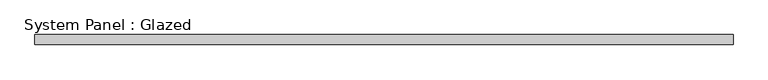
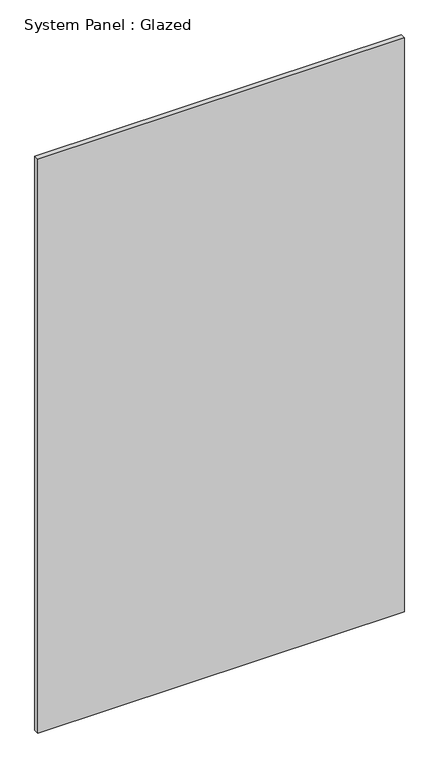
"""IFC4 building model written with IfcOpenShell, lengths in millimetres: plate geometry, System Panel : Glazed."""

from ifc_helpers import new_model, si_unit, origin, origin_with_axes, place, context, project, spatial, polyline, outline, extrude, source, transform, mapped, element, save


def system_panel_glazed_10fc8cc6(model_context):
    return source(origin(), model_context, "Body", "SweptSolid", [
        extrude(outline(polyline([(882.65, -44.45), (-882.65, -44.45), (-882.65, -19.05), (882.65, -19.05), (882.65, -44.45)])), origin_with_axes(), (0.0, 0.0, 1.0), 2921.0),
    ])


if __name__ == "__main__":
    model = new_model("IFC4")
    model_context = context("Model", 3, world=origin())
    ifc_project = project(units=[si_unit("LENGTHUNIT", "METRE", prefix="MILLI")], contexts=[model_context])
    site = spatial("IfcSite", under=ifc_project)
    building = spatial("IfcBuilding", under=site)
    placement = place(None, origin())
    system_panel_glazed_shape = system_panel_glazed_10fc8cc6(model_context)
    element("IfcPlate", 1, ObjectType="System Panel : Glazed", at=placement, inside=building, context=model_context, shape_type="MappedRepresentation", body=[
        mapped(system_panel_glazed_shape, transform((0.0, 0.0, 0.0), x_axis=(1.0, 0.0, 0.0), y_axis=(0.0, 1.0, 0.0), z_axis=(0.0, 0.0, 1.0))),
    ])
    save(model, "model.ifc")

# Revit data of these elements
# Type "System Panel : Glazed"
#   Construction Type Id = "GSP4R"
#   Analytic Construction = "1/8 in Pilkington single glazing"
#   Visual Light Transmittance = 0.9
#   Solar Heat Gain Coefficient = 0.86
#   Heat Transfer Coefficient (U) = 1.18115 BTU/(h·ft²·°F)
# Element 1 (IfcPlate, "System Panel : Glazed")
#   Materials on its faces: "Glass"
# Materials
#   "Glass": class "Glass", colour RGB 0 128 192, transparency 0.75, Description = "Soda Lime Glass", Cost = 0
